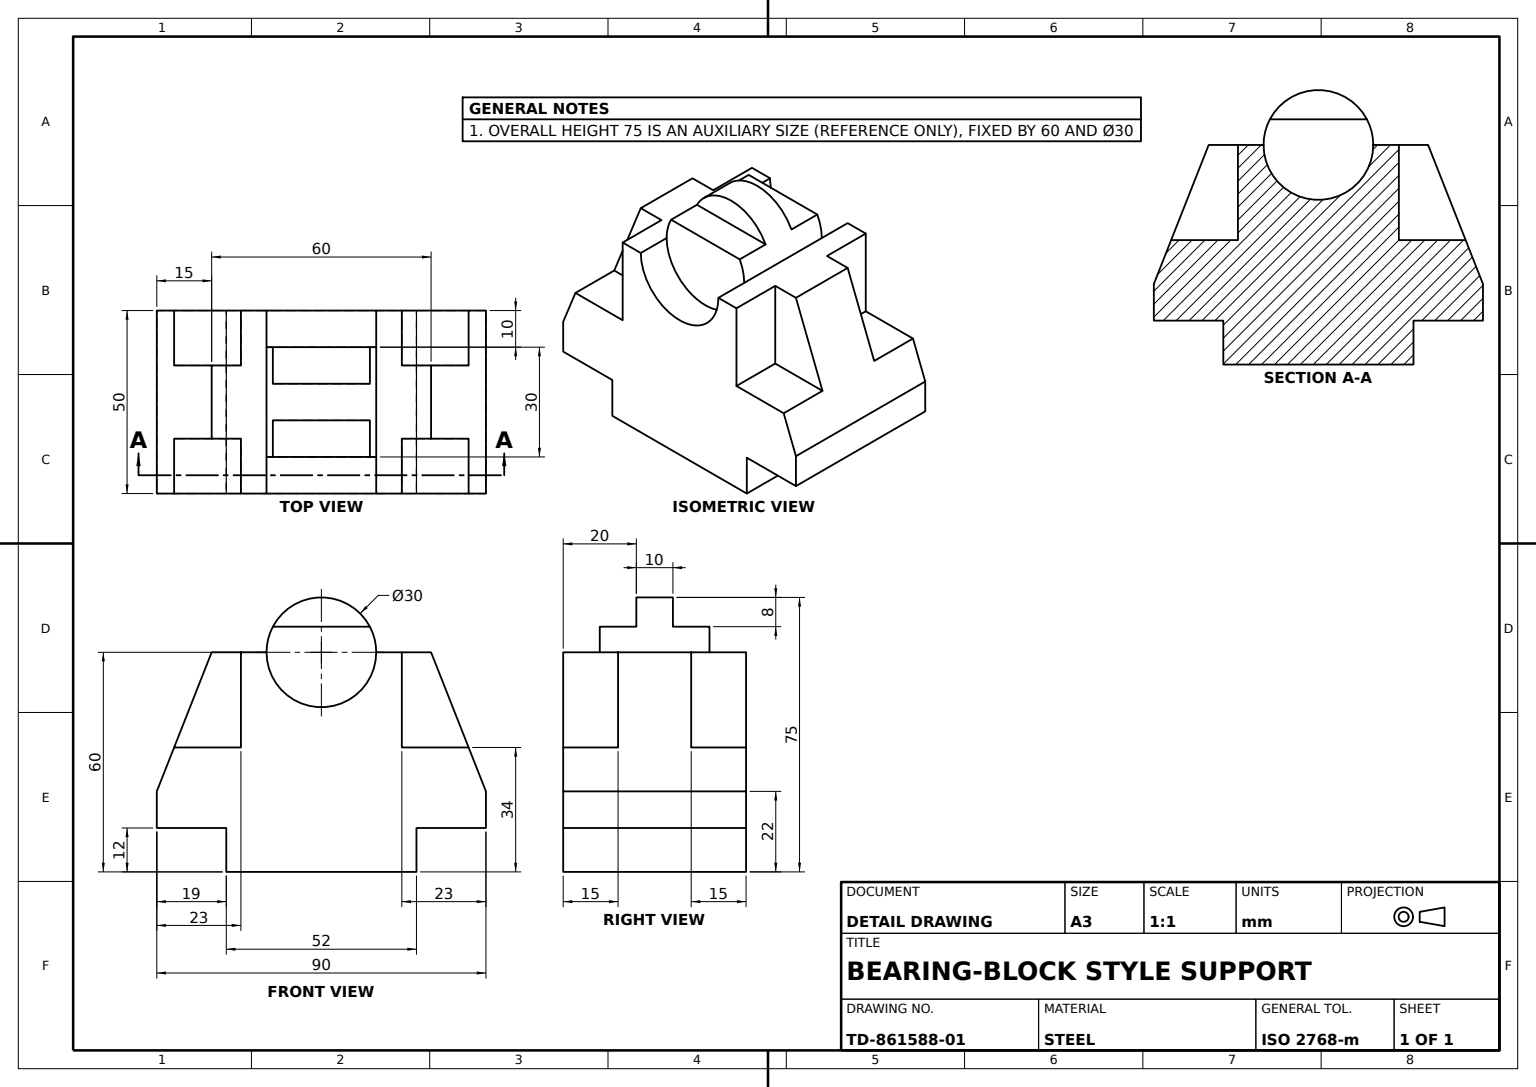
from build123d import *

# Parameters (mm, degrees)
SADDLE_BODY_DEPTH                      = 25
CORNER_POCKET_34X22_DEPTH              = 15
CORNER_POCKET_MIRROR_SIDE_COPY_1_DEPTH = 15
BORE_SKETCH_R                          = 15
BORE_30_DEPTH                          = 83.637763765
BORE_PLUG_SKETCH_R                     = 15
BORE_PLUG_DEPTH                        = 15
PLUG_SLOT_SKETCH_W                     = 10
PLUG_SLOT_SKETCH_H                     = 8
PLUG_SLOT_8X10_DEPTH                   = 15


with BuildPart() as part:
    # Saddle Profile Sketch → Saddle Body (new, symmetric)
    with BuildSketch(Plane.XY):
        Polygon((-45, 0), (-45, 10), (-30, 48), (30, 48), (45, 10), (45, 0), (26, 0), (26, -12), (-26, -12), (-26, 0), align=None)
    extrude(amount=SADDLE_BODY_DEPTH, both=True)

    # Corner Pocket Sketch → Corner Pocket 34x22 (cut)
    with BuildSketch(Plane.XY.offset(25)):
        Polygon((-30, 48), (-22, 48), (-22, 22), (-40.263157895, 22), align=None)
    corner_pocket_34x22 = extrude(amount=-CORNER_POCKET_34X22_DEPTH, mode=Mode.SUBTRACT)

    # Corner Pocket Mirror Front: Corner Pocket 34x22 across plane
    add(corner_pocket_34x22.mirror(Plane.XY), mode=Mode.SUBTRACT)

    # Corner Pocket Mirror Side: Corner Pocket 34x22 across plane
    add(corner_pocket_34x22.mirror(Plane(origin=(0, 0, 0), x_dir=(0, 0, 1), z_dir=(1, 0, 0))), mode=Mode.SUBTRACT)

    # Corner Pocket Mirror Side copy 1 sketch → Corner Pocket Mirror Side copy 1 (cut)
    with BuildSketch(Plane(origin=(0, 0, -25), x_dir=(-1, 0, 0), z_dir=(0, 0, -1))):
        Polygon((-30, 48), (-22, 48), (-22, 22), (-40.263157895, 22), align=None)
    extrude(amount=-CORNER_POCKET_MIRROR_SIDE_COPY_1_DEPTH, mode=Mode.SUBTRACT)

    # Bore Sketch → Bore Ø30 (cut, through all)
    with BuildSketch(Plane.XY.offset(25)):
        with Locations((0, 48)):
            Circle(BORE_SKETCH_R)
    extrude(amount=-BORE_30_DEPTH, mode=Mode.SUBTRACT)

    # Bore Plug Sketch → Bore Plug (add, symmetric)
    with BuildSketch(Plane.XY):
        with Locations((0, 48)):
            Circle(BORE_PLUG_SKETCH_R)
    extrude(amount=BORE_PLUG_DEPTH, both=True)

    # Plug Slot Sketch → Plug Slot 8x10 (cut, symmetric)
    with BuildSketch(Plane(origin=(0, 0, 0), x_dir=(0, 0, -1), z_dir=(1, 0, 0))):
        with Locations((10, 59)):
            Rectangle(PLUG_SLOT_SKETCH_W, PLUG_SLOT_SKETCH_H)
    plug_slot_8x10 = extrude(amount=PLUG_SLOT_8X10_DEPTH, both=True, mode=Mode.SUBTRACT)

    # Plug Slot Mirror: Plug Slot 8x10 across plane
    add(plug_slot_8x10.mirror(Plane.XY), mode=Mode.SUBTRACT)


solid = part.part
